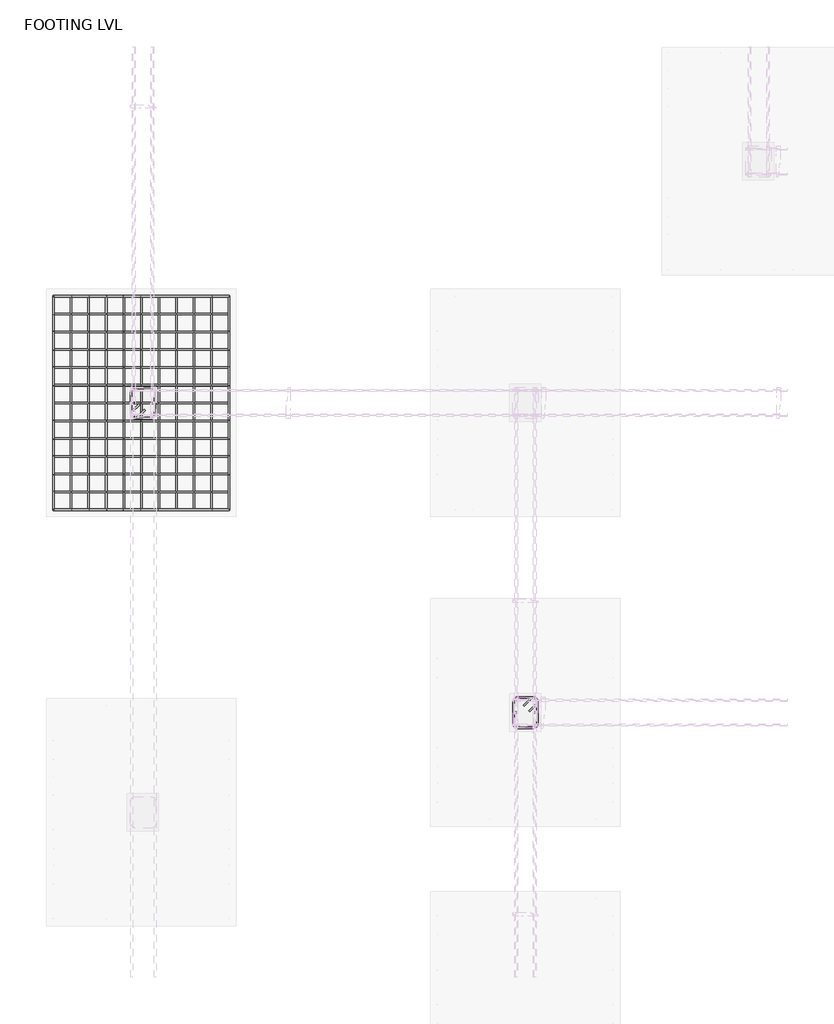
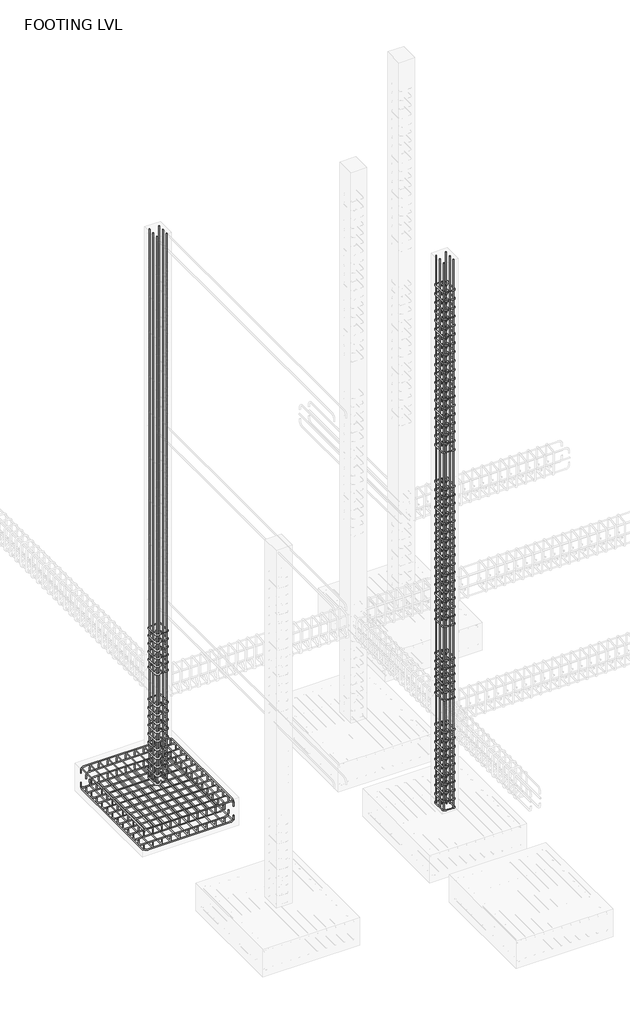
# One storey, part 4 of 16: 22 reinforcing bars.
"""IFC4 building model written with IfcOpenShell, lengths in millimetres."""

from ifc_helpers import new_model, si_unit, point, frame, origin, place, context, project, spatial, polyline, circle_curve, trimmed, segment, composite_curve, source, transform, mapped, element, save
from ifc_brep_helpers import swept_disk

model = new_model("IFC4")

# Units and contexts
model_context = context("Model", 3, world=origin())
ifc_project = project(units=[si_unit("LENGTHUNIT", "METRE", prefix="MILLI")], contexts=[model_context])

# Site, building, storey
site = spatial("IfcSite", under=ifc_project)
building = spatial("IfcBuilding", under=site)
storey = spatial("IfcBuildingStorey", under=building, Name="FOOTING LVL", Elevation=-1828.8)

# Reinforcing bars
placement = place(None, origin())
reinforcing_bar_shape = source(origin(), model_context, "Body", "SolidModel", [
    swept_disk(composite_curve([segment(polyline([(-13401.9759067, 5358.4372759, -2134.39375), (-13401.9759067, 5358.4372759, -2185.19375)]), True, "CONTINUOUS"), segment(trimmed(circle_curve(frame((-13357.5259067, 5358.4372759, -2185.19375), z_axis=(0.0, -1.0, 0.0), x_axis=(-44.44999999999891, 0.0, 0.0)), 44.45), [point((-13401.9759067, 5358.4372759, -2185.19375))], [point((-13357.5259067, 5358.4372759, -2229.64375))], True, "CARTESIAN"), True, "CONTINUOUS"), segment(polyline([(-13357.5259067, 5358.4372759, -2229.64375), (-12035.1384067, 5358.4372759, -2229.64375)]), True, "CONTINUOUS"), segment(trimmed(circle_curve(frame((-12035.1384067, 5358.4372759, -2185.19375), z_axis=(0.0, -1.0, 0.0), x_axis=(0.0, 0.0, -44.45000000000027)), 44.45), [point((-12035.1384067, 5358.4372759, -2229.64375))], [point((-11990.6884067, 5358.4372759, -2185.19375))], True, "CARTESIAN"), True, "CONTINUOUS"), segment(polyline([(-11990.6884067, 5358.4372759, -2185.19375), (-11990.6884067, 5358.4372759, -2134.39375)]), True, "CONTINUOUS")], self_intersect=False), 6.35),
])
element("IfcReinforcingBar", 1, at=placement, inside=storey, context=model_context, shape_type="MappedRepresentation", body=[
    mapped(reinforcing_bar_shape, transform((0.0, 0.0, 0.0), x_axis=(1.0, 0.0, 0.0), y_axis=(0.0, 1.0, 0.0), z_axis=(0.0, 0.0, 1.0))),
    mapped(reinforcing_bar_shape, transform((0.0, 143.0072917, 0.0), x_axis=(1.0, 0.0, 0.0), y_axis=(0.0, 1.0, 0.0), z_axis=(0.0, 0.0, 1.0))),
    mapped(reinforcing_bar_shape, transform((0.0, 286.0145833, 0.0), x_axis=(1.0, 0.0, 0.0), y_axis=(0.0, 1.0, 0.0), z_axis=(0.0, 0.0, 1.0))),
    mapped(reinforcing_bar_shape, transform((0.0, 429.021875, 0.0), x_axis=(1.0, 0.0, 0.0), y_axis=(0.0, 1.0, 0.0), z_axis=(0.0, 0.0, 1.0))),
    mapped(reinforcing_bar_shape, transform((0.0, 572.0291667, 0.0), x_axis=(1.0, 0.0, 0.0), y_axis=(0.0, 1.0, 0.0), z_axis=(0.0, 0.0, 1.0))),
    mapped(reinforcing_bar_shape, transform((0.0, 715.0364583, 0.0), x_axis=(1.0, 0.0, 0.0), y_axis=(0.0, 1.0, 0.0), z_axis=(0.0, 0.0, 1.0))),
    mapped(reinforcing_bar_shape, transform((0.0, 858.04375, 0.0), x_axis=(1.0, 0.0, 0.0), y_axis=(0.0, 1.0, 0.0), z_axis=(0.0, 0.0, 1.0))),
    mapped(reinforcing_bar_shape, transform((0.0, 1001.0510417, 0.0), x_axis=(1.0, 0.0, 0.0), y_axis=(0.0, 1.0, 0.0), z_axis=(0.0, 0.0, 1.0))),
    mapped(reinforcing_bar_shape, transform((0.0, 1144.0583333, 0.0), x_axis=(1.0, 0.0, 0.0), y_axis=(0.0, 1.0, 0.0), z_axis=(0.0, 0.0, 1.0))),
    mapped(reinforcing_bar_shape, transform((0.0, 1287.065625, 0.0), x_axis=(1.0, 0.0, 0.0), y_axis=(0.0, 1.0, 0.0), z_axis=(0.0, 0.0, 1.0))),
    mapped(reinforcing_bar_shape, transform((0.0, 1430.0729167, 0.0), x_axis=(1.0, 0.0, 0.0), y_axis=(0.0, 1.0, 0.0), z_axis=(0.0, 0.0, 1.0))),
    mapped(reinforcing_bar_shape, transform((0.0, 1573.0802083, 0.0), x_axis=(1.0, 0.0, 0.0), y_axis=(0.0, 1.0, 0.0), z_axis=(0.0, 0.0, 1.0))),
    mapped(reinforcing_bar_shape, transform((0.0, 1716.0875, 0.0), x_axis=(1.0, 0.0, 0.0), y_axis=(0.0, 1.0, 0.0), z_axis=(0.0, 0.0, 1.0))),
])
reinforcing_bar_2_shape = source(origin(), model_context, "Body", "SolidModel", [
    swept_disk(composite_curve([segment(polyline([(-11990.6884067, 5358.4372759, -1980.40625), (-11990.6884067, 5358.4372759, -1929.60625)]), True, "CONTINUOUS"), segment(trimmed(circle_curve(frame((-12035.1384067, 5358.4372759, -1929.60625), z_axis=(0.0, -1.0, 0.0), x_axis=(44.45000000000073, 0.0, 0.0)), 44.45), [point((-11990.6884067, 5358.4372759, -1929.60625))], [point((-12035.1384067, 5358.4372759, -1885.15625))], True, "CARTESIAN"), True, "CONTINUOUS"), segment(polyline([(-12035.1384067, 5358.4372759, -1885.15625), (-13357.5259067, 5358.4372759, -1885.15625)]), True, "CONTINUOUS"), segment(trimmed(circle_curve(frame((-13357.5259067, 5358.4372759, -1929.60625), z_axis=(0.0, -1.0, 0.0), x_axis=(0.0, 0.0, 44.450000000000045)), 44.45), [point((-13357.5259067, 5358.4372759, -1885.15625))], [point((-13401.9759067, 5358.4372759, -1929.60625))], True, "CARTESIAN"), True, "CONTINUOUS"), segment(polyline([(-13401.9759067, 5358.4372759, -1929.60625), (-13401.9759067, 5358.4372759, -1980.40625)]), True, "CONTINUOUS")], self_intersect=False), 6.35),
])
element("IfcReinforcingBar", 2, at=placement, inside=storey, context=model_context, shape_type="MappedRepresentation", body=[
    mapped(reinforcing_bar_2_shape, transform((0.0, 0.0, 0.0), x_axis=(1.0, 0.0, 0.0), y_axis=(0.0, 1.0, 0.0), z_axis=(0.0, 0.0, 1.0))),
    mapped(reinforcing_bar_2_shape, transform((0.0, 143.0072917, 0.0), x_axis=(1.0, 0.0, 0.0), y_axis=(0.0, 1.0, 0.0), z_axis=(0.0, 0.0, 1.0))),
    mapped(reinforcing_bar_2_shape, transform((0.0, 286.0145833, 0.0), x_axis=(1.0, 0.0, 0.0), y_axis=(0.0, 1.0, 0.0), z_axis=(0.0, 0.0, 1.0))),
    mapped(reinforcing_bar_2_shape, transform((0.0, 429.021875, 0.0), x_axis=(1.0, 0.0, 0.0), y_axis=(0.0, 1.0, 0.0), z_axis=(0.0, 0.0, 1.0))),
    mapped(reinforcing_bar_2_shape, transform((0.0, 572.0291667, 0.0), x_axis=(1.0, 0.0, 0.0), y_axis=(0.0, 1.0, 0.0), z_axis=(0.0, 0.0, 1.0))),
    mapped(reinforcing_bar_2_shape, transform((0.0, 715.0364583, 0.0), x_axis=(1.0, 0.0, 0.0), y_axis=(0.0, 1.0, 0.0), z_axis=(0.0, 0.0, 1.0))),
    mapped(reinforcing_bar_2_shape, transform((0.0, 858.04375, 0.0), x_axis=(1.0, 0.0, 0.0), y_axis=(0.0, 1.0, 0.0), z_axis=(0.0, 0.0, 1.0))),
    mapped(reinforcing_bar_2_shape, transform((0.0, 1001.0510417, 0.0), x_axis=(1.0, 0.0, 0.0), y_axis=(0.0, 1.0, 0.0), z_axis=(0.0, 0.0, 1.0))),
    mapped(reinforcing_bar_2_shape, transform((0.0, 1144.0583333, 0.0), x_axis=(1.0, 0.0, 0.0), y_axis=(0.0, 1.0, 0.0), z_axis=(0.0, 0.0, 1.0))),
    mapped(reinforcing_bar_2_shape, transform((0.0, 1287.065625, 0.0), x_axis=(1.0, 0.0, 0.0), y_axis=(0.0, 1.0, 0.0), z_axis=(0.0, 0.0, 1.0))),
    mapped(reinforcing_bar_2_shape, transform((0.0, 1430.0729167, 0.0), x_axis=(1.0, 0.0, 0.0), y_axis=(0.0, 1.0, 0.0), z_axis=(0.0, 0.0, 1.0))),
    mapped(reinforcing_bar_2_shape, transform((0.0, 1573.0802083, 0.0), x_axis=(1.0, 0.0, 0.0), y_axis=(0.0, 1.0, 0.0), z_axis=(0.0, 0.0, 1.0))),
    mapped(reinforcing_bar_2_shape, transform((0.0, 1716.0875, 0.0), x_axis=(1.0, 0.0, 0.0), y_axis=(0.0, 1.0, 0.0), z_axis=(0.0, 0.0, 1.0))),
])
reinforcing_bar_3_shape = source(origin(), model_context, "Body", "SolidModel", [
    swept_disk(composite_curve([segment(polyline([(-11990.6884067, 7074.5247759, -1980.40625), (-11990.6884067, 7074.5247759, -1929.60625)]), True, "CONTINUOUS"), segment(trimmed(circle_curve(frame((-11990.6884067, 7030.0747759, -1929.60625), z_axis=(1.0, 0.0, 0.0), x_axis=(0.0, 44.45000000000073, 0.0)), 44.45), [point((-11990.6884067, 7074.5247759, -1929.60625))], [point((-11990.6884067, 7030.0747759, -1885.15625))], True, "CARTESIAN"), True, "CONTINUOUS"), segment(polyline([(-11990.6884067, 7030.0747759, -1885.15625), (-11990.6884067, 5402.8872759, -1885.15625)]), True, "CONTINUOUS"), segment(trimmed(circle_curve(frame((-11990.6884067, 5402.8872759, -1929.60625), z_axis=(1.0, 0.0, 0.0), x_axis=(0.0, 0.0, 44.450000000000045)), 44.45), [point((-11990.6884067, 5402.8872759, -1885.15625))], [point((-11990.6884067, 5358.4372759, -1929.60625))], True, "CARTESIAN"), True, "CONTINUOUS"), segment(polyline([(-11990.6884067, 5358.4372759, -1929.60625), (-11990.6884067, 5358.4372759, -1980.40625)]), True, "CONTINUOUS")], self_intersect=False), 6.35),
])
element("IfcReinforcingBar", 3, at=placement, inside=storey, context=model_context, shape_type="MappedRepresentation", body=[
    mapped(reinforcing_bar_3_shape, transform((0.0, 0.0, 0.0), x_axis=(1.0, 0.0, 0.0), y_axis=(0.0, 1.0, 0.0), z_axis=(0.0, 0.0, 1.0))),
    mapped(reinforcing_bar_3_shape, transform((-141.12875, 0.0, 0.0), x_axis=(1.0, 0.0, 0.0), y_axis=(0.0, 1.0, 0.0), z_axis=(0.0, 0.0, 1.0))),
    mapped(reinforcing_bar_3_shape, transform((-282.2575, 0.0, 0.0), x_axis=(1.0, 0.0, 0.0), y_axis=(0.0, 1.0, 0.0), z_axis=(0.0, 0.0, 1.0))),
    mapped(reinforcing_bar_3_shape, transform((-423.38625, 0.0, 0.0), x_axis=(1.0, 0.0, 0.0), y_axis=(0.0, 1.0, 0.0), z_axis=(0.0, 0.0, 1.0))),
    mapped(reinforcing_bar_3_shape, transform((-564.515, 0.0, 0.0), x_axis=(1.0, 0.0, 0.0), y_axis=(0.0, 1.0, 0.0), z_axis=(0.0, 0.0, 1.0))),
    mapped(reinforcing_bar_3_shape, transform((-705.64375, 0.0, 0.0), x_axis=(1.0, 0.0, 0.0), y_axis=(0.0, 1.0, 0.0), z_axis=(0.0, 0.0, 1.0))),
    mapped(reinforcing_bar_3_shape, transform((-846.7725, 0.0, 0.0), x_axis=(1.0, 0.0, 0.0), y_axis=(0.0, 1.0, 0.0), z_axis=(0.0, 0.0, 1.0))),
    mapped(reinforcing_bar_3_shape, transform((-987.90125, 0.0, 0.0), x_axis=(1.0, 0.0, 0.0), y_axis=(0.0, 1.0, 0.0), z_axis=(0.0, 0.0, 1.0))),
    mapped(reinforcing_bar_3_shape, transform((-1129.03, 0.0, 0.0), x_axis=(1.0, 0.0, 0.0), y_axis=(0.0, 1.0, 0.0), z_axis=(0.0, 0.0, 1.0))),
    mapped(reinforcing_bar_3_shape, transform((-1270.15875, 0.0, 0.0), x_axis=(1.0, 0.0, 0.0), y_axis=(0.0, 1.0, 0.0), z_axis=(0.0, 0.0, 1.0))),
    mapped(reinforcing_bar_3_shape, transform((-1411.2875, 0.0, 0.0), x_axis=(1.0, 0.0, 0.0), y_axis=(0.0, 1.0, 0.0), z_axis=(0.0, 0.0, 1.0))),
])
reinforcing_bar_4_shape = source(origin(), model_context, "Body", "SolidModel", [
    swept_disk(composite_curve([segment(polyline([(-13401.9759067, 7074.5247759, -2134.39375), (-13401.9759067, 7074.5247759, -2185.19375)]), True, "CONTINUOUS"), segment(trimmed(circle_curve(frame((-13401.9759067, 7030.0747759, -2185.19375), z_axis=(-1.0, 0.0, 0.0), x_axis=(0.0, 44.45000000000073, 0.0)), 44.45), [point((-13401.9759067, 7074.5247759, -2185.19375))], [point((-13401.9759067, 7030.0747759, -2229.64375))], True, "CARTESIAN"), True, "CONTINUOUS"), segment(polyline([(-13401.9759067, 7030.0747759, -2229.64375), (-13401.9759067, 5402.8872759, -2229.64375)]), True, "CONTINUOUS"), segment(trimmed(circle_curve(frame((-13401.9759067, 5402.8872759, -2185.19375), z_axis=(-1.0, 0.0, 0.0), x_axis=(0.0, 0.0, -44.45000000000027)), 44.45), [point((-13401.9759067, 5402.8872759, -2229.64375))], [point((-13401.9759067, 5358.4372759, -2185.19375))], True, "CARTESIAN"), True, "CONTINUOUS"), segment(polyline([(-13401.9759067, 5358.4372759, -2185.19375), (-13401.9759067, 5358.4372759, -2134.39375)]), True, "CONTINUOUS")], self_intersect=False), 6.35),
])
element("IfcReinforcingBar", 4, at=placement, inside=storey, context=model_context, shape_type="MappedRepresentation", body=[
    mapped(reinforcing_bar_4_shape, transform((0.0, 0.0, 0.0), x_axis=(1.0, 0.0, 0.0), y_axis=(0.0, 1.0, 0.0), z_axis=(0.0, 0.0, 1.0))),
    mapped(reinforcing_bar_4_shape, transform((141.12875, 0.0, 0.0), x_axis=(1.0, 0.0, 0.0), y_axis=(0.0, 1.0, 0.0), z_axis=(0.0, 0.0, 1.0))),
    mapped(reinforcing_bar_4_shape, transform((282.2575, 0.0, 0.0), x_axis=(1.0, 0.0, 0.0), y_axis=(0.0, 1.0, 0.0), z_axis=(0.0, 0.0, 1.0))),
    mapped(reinforcing_bar_4_shape, transform((423.38625, 0.0, 0.0), x_axis=(1.0, 0.0, 0.0), y_axis=(0.0, 1.0, 0.0), z_axis=(0.0, 0.0, 1.0))),
    mapped(reinforcing_bar_4_shape, transform((564.515, 0.0, 0.0), x_axis=(1.0, 0.0, 0.0), y_axis=(0.0, 1.0, 0.0), z_axis=(0.0, 0.0, 1.0))),
    mapped(reinforcing_bar_4_shape, transform((705.64375, 0.0, 0.0), x_axis=(1.0, 0.0, 0.0), y_axis=(0.0, 1.0, 0.0), z_axis=(0.0, 0.0, 1.0))),
    mapped(reinforcing_bar_4_shape, transform((846.7725, 0.0, 0.0), x_axis=(1.0, 0.0, 0.0), y_axis=(0.0, 1.0, 0.0), z_axis=(0.0, 0.0, 1.0))),
    mapped(reinforcing_bar_4_shape, transform((987.90125, 0.0, 0.0), x_axis=(1.0, 0.0, 0.0), y_axis=(0.0, 1.0, 0.0), z_axis=(0.0, 0.0, 1.0))),
    mapped(reinforcing_bar_4_shape, transform((1129.03, 0.0, 0.0), x_axis=(1.0, 0.0, 0.0), y_axis=(0.0, 1.0, 0.0), z_axis=(0.0, 0.0, 1.0))),
    mapped(reinforcing_bar_4_shape, transform((1270.15875, 0.0, 0.0), x_axis=(1.0, 0.0, 0.0), y_axis=(0.0, 1.0, 0.0), z_axis=(0.0, 0.0, 1.0))),
    mapped(reinforcing_bar_4_shape, transform((1411.2875, 0.0, 0.0), x_axis=(1.0, 0.0, 0.0), y_axis=(0.0, 1.0, 0.0), z_axis=(0.0, 0.0, 1.0))),
])
reinforcing_bar_5_shape = source(origin(), model_context, "Body", "SolidModel", [
    swept_disk(composite_curve([segment(polyline([(-12714.355274, 6204.4997897, -1797.446875), (-12769.2202725, 6149.6347912, -1797.446875)]), True, "CONTINUOUS"), segment(trimmed(circle_curve(frame((-12746.7696322, 6127.1841509, -1797.446875), z_axis=(0.0, 0.0, 1.0), x_axis=(-22.450640300001396, 22.450640300000487, 0.0)), 31.75), [point((-12769.2202725, 6149.6347912, -1797.446875))], [point((-12746.7696322, 6095.4341509, -1797.446875))], True, "CARTESIAN"), True, "CONTINUOUS"), segment(polyline([(-12746.7696322, 6095.4341509, -1797.446875), (-12618.9758822, 6095.4341509, -1797.446875)]), True, "CONTINUOUS"), segment(trimmed(circle_curve(frame((-12618.9758822, 6127.1841509, -1797.446875), z_axis=(0.0, 0.0, 1.0), x_axis=(0.0, -31.75, 0.0)), 31.75), [point((-12618.9758822, 6095.4341509, -1797.446875))], [point((-12587.2258822, 6127.1841509, -1797.446875))], True, "CARTESIAN"), True, "CONTINUOUS"), segment(polyline([(-12587.2258822, 6127.1841509, -1797.446875), (-12587.2258822, 6305.7779009, -1797.446875)]), True, "CONTINUOUS"), segment(trimmed(circle_curve(frame((-12618.9061414, 6305.7779009, -1799.5501287), z_axis=(-0.06624421176864072, 0.0, 0.9978034397651431), x_axis=(31.680259200000364, 0.0, 2.1032536999998683)), 31.75), [point((-12587.2258822, 6305.7779009, -1797.446875))], [point((-12618.9061414, 6337.5279009, -1799.5501287))], True, "CARTESIAN"), True, "CONTINUOUS"), segment(polyline([(-12618.9061414, 6337.5279009, -1799.5501287), (-12746.839373, 6337.5279009, -1808.0436213)]), True, "CONTINUOUS"), segment(trimmed(circle_curve(frame((-12746.839373, 6305.7779009, -1808.0436213), z_axis=(-0.06624421176864072, 0.0, 0.9978034397651431), x_axis=(0.0, 31.75, 0.0)), 31.75), [point((-12746.839373, 6337.5279009, -1808.0436213))], [point((-12778.5196322, 6305.7779009, -1810.146875))], True, "CARTESIAN"), True, "CONTINUOUS"), segment(polyline([(-12778.5196322, 6305.7779009, -1810.146875), (-12778.5196322, 6127.1841509, -1810.146875)]), True, "CONTINUOUS"), segment(trimmed(circle_curve(frame((-12746.7696322, 6127.1841509, -1810.146875), z_axis=(0.0, 0.0, 1.0), x_axis=(-31.75, 0.0, 0.0)), 31.75), [point((-12778.5196322, 6127.1841509, -1810.146875))], [point((-12724.3189919, 6104.7335106, -1810.146875))], True, "CARTESIAN"), True, "CONTINUOUS"), segment(polyline([(-12724.3189919, 6104.7335106, -1810.146875), (-12669.4539934, 6159.5985091, -1810.146875)]), True, "CONTINUOUS")], self_intersect=False), 6.35),
])
element("IfcReinforcingBar", 5, at=placement, inside=storey, context=model_context, shape_type="MappedRepresentation", body=[
    mapped(reinforcing_bar_5_shape, transform((0.0, 0.0, 0.0), x_axis=(1.0, 0.0, 0.0), y_axis=(0.0, 1.0, 0.0), z_axis=(0.0, 0.0, 1.0))),
    mapped(reinforcing_bar_5_shape, transform((0.0, 0.0, 144.2276574), x_axis=(1.0, 0.0, 0.0), y_axis=(0.0, 1.0, 0.0), z_axis=(0.0, 0.0, 1.0))),
    mapped(reinforcing_bar_5_shape, transform((0.0, 0.0, 288.4553149), x_axis=(1.0, 0.0, 0.0), y_axis=(0.0, 1.0, 0.0), z_axis=(0.0, 0.0, 1.0))),
    mapped(reinforcing_bar_5_shape, transform((0.0, 0.0, 432.6829723), x_axis=(1.0, 0.0, 0.0), y_axis=(0.0, 1.0, 0.0), z_axis=(0.0, 0.0, 1.0))),
    mapped(reinforcing_bar_5_shape, transform((0.0, 0.0, 576.9106298), x_axis=(1.0, 0.0, 0.0), y_axis=(0.0, 1.0, 0.0), z_axis=(0.0, 0.0, 1.0))),
    mapped(reinforcing_bar_5_shape, transform((0.0, 0.0, 721.1382872), x_axis=(1.0, 0.0, 0.0), y_axis=(0.0, 1.0, 0.0), z_axis=(0.0, 0.0, 1.0))),
    mapped(reinforcing_bar_5_shape, transform((0.0, 0.0, 865.3659446), x_axis=(1.0, 0.0, 0.0), y_axis=(0.0, 1.0, 0.0), z_axis=(0.0, 0.0, 1.0))),
    mapped(reinforcing_bar_5_shape, transform((0.0, 0.0, 1009.5936021), x_axis=(1.0, 0.0, 0.0), y_axis=(0.0, 1.0, 0.0), z_axis=(0.0, 0.0, 1.0))),
    mapped(reinforcing_bar_5_shape, transform((0.0, 0.0, 1153.8212595), x_axis=(1.0, 0.0, 0.0), y_axis=(0.0, 1.0, 0.0), z_axis=(0.0, 0.0, 1.0))),
    mapped(reinforcing_bar_5_shape, transform((0.0, 0.0, 1298.048917), x_axis=(1.0, 0.0, 0.0), y_axis=(0.0, 1.0, 0.0), z_axis=(0.0, 0.0, 1.0))),
])
element("IfcReinforcingBar", 6, at=placement, inside=storey, context=model_context, shape_type="SolidModel", body=[
    swept_disk(composite_curve([segment(polyline([(-12760.2400164, 6113.7137667, -1803.796875), (-12760.2400164, 6113.7137667, 7290.196875)]), True, "CONTINUOUS")], self_intersect=False), 6.35),
])
element("IfcReinforcingBar", 7, at=placement, inside=storey, context=model_context, shape_type="SolidModel", body=[
    swept_disk(composite_curve([segment(polyline([(-12605.505498, 6113.7137667, -1803.796875), (-12605.505498, 6113.7137667, 7290.196875)]), True, "CONTINUOUS")], self_intersect=False), 6.35),
])
element("IfcReinforcingBar", 8, at=placement, inside=storey, context=model_context, shape_type="SolidModel", body=[
    swept_disk(composite_curve([segment(polyline([(-12760.2400164, 6319.2482851, -1803.796875), (-12760.2400164, 6319.2482851, 7290.196875)]), True, "CONTINUOUS")], self_intersect=False), 6.35),
])
element("IfcReinforcingBar", 9, at=placement, inside=storey, context=model_context, shape_type="SolidModel", body=[
    swept_disk(composite_curve([segment(polyline([(-12605.505498, 6319.2482851, -1803.796875), (-12605.505498, 6319.2482851, 7290.196875)]), True, "CONTINUOUS")], self_intersect=False), 6.35),
])
element("IfcReinforcingBar", 10, at=placement, inside=storey, context=model_context, shape_type="SolidModel", body=[
    swept_disk(composite_curve([segment(polyline([(-12760.2400164, 6216.4810259, -1803.796875), (-12760.2400164, 6216.4810259, 7290.196875)]), True, "CONTINUOUS")], self_intersect=False), 6.35),
])
element("IfcReinforcingBar", 11, at=placement, inside=storey, context=model_context, shape_type="SolidModel", body=[
    swept_disk(composite_curve([segment(polyline([(-12605.505498, 6216.4810259, -1803.796875), (-12605.505498, 6216.4810259, 7290.196875)]), True, "CONTINUOUS")], self_intersect=False), 6.35),
])
reinforcing_bar_6_shape = source(origin(), model_context, "Body", "SolidModel", [
    swept_disk(composite_curve([segment(polyline([(-12714.355274, 6204.4997897, 31.353125), (-12769.2202725, 6149.6347912, 31.353125)]), True, "CONTINUOUS"), segment(trimmed(circle_curve(frame((-12746.7696322, 6127.1841509, 31.353125), z_axis=(0.0, 0.0, 1.0), x_axis=(-22.450640300001396, 22.450640300000487, 0.0)), 31.75), [point((-12769.2202725, 6149.6347912, 31.353125))], [point((-12746.7696322, 6095.4341509, 31.353125))], True, "CARTESIAN"), True, "CONTINUOUS"), segment(polyline([(-12746.7696322, 6095.4341509, 31.353125), (-12618.9758822, 6095.4341509, 31.353125)]), True, "CONTINUOUS"), segment(trimmed(circle_curve(frame((-12618.9758822, 6127.1841509, 31.353125), z_axis=(0.0, 0.0, 1.0), x_axis=(0.0, -31.75, 0.0)), 31.75), [point((-12618.9758822, 6095.4341509, 31.353125))], [point((-12587.2258822, 6127.1841509, 31.353125))], True, "CARTESIAN"), True, "CONTINUOUS"), segment(polyline([(-12587.2258822, 6127.1841509, 31.353125), (-12587.2258822, 6305.7779009, 31.353125)]), True, "CONTINUOUS"), segment(trimmed(circle_curve(frame((-12618.9061414, 6305.7779009, 29.2498713), z_axis=(-0.06624421176864072, 0.0, 0.9978034397651431), x_axis=(31.680259200000364, 0.0, 2.1032537)), 31.75), [point((-12587.2258822, 6305.7779009, 31.353125))], [point((-12618.9061414, 6337.5279009, 29.2498713))], True, "CARTESIAN"), True, "CONTINUOUS"), segment(polyline([(-12618.9061414, 6337.5279009, 29.2498713), (-12746.839373, 6337.5279009, 20.7563787)]), True, "CONTINUOUS"), segment(trimmed(circle_curve(frame((-12746.839373, 6305.7779009, 20.7563787), z_axis=(-0.06624421176864072, 0.0, 0.9978034397651431), x_axis=(0.0, 31.75, 0.0)), 31.75), [point((-12746.839373, 6337.5279009, 20.7563787))], [point((-12778.5196322, 6305.7779009, 18.653125))], True, "CARTESIAN"), True, "CONTINUOUS"), segment(polyline([(-12778.5196322, 6305.7779009, 18.653125), (-12778.5196322, 6127.1841509, 18.653125)]), True, "CONTINUOUS"), segment(trimmed(circle_curve(frame((-12746.7696322, 6127.1841509, 18.653125), z_axis=(0.0, 0.0, 1.0), x_axis=(-31.75, 0.0, 0.0)), 31.75), [point((-12778.5196322, 6127.1841509, 18.653125))], [point((-12724.3189919, 6104.7335106, 18.653125))], True, "CARTESIAN"), True, "CONTINUOUS"), segment(polyline([(-12724.3189919, 6104.7335106, 18.653125), (-12669.4539934, 6159.5985091, 18.653125)]), True, "CONTINUOUS")], self_intersect=False), 6.35),
])
element("IfcReinforcingBar", 12, at=placement, inside=storey, context=model_context, shape_type="MappedRepresentation", body=[
    mapped(reinforcing_bar_6_shape, transform((0.0, 0.0, 0.0), x_axis=(1.0, 0.0, 0.0), y_axis=(0.0, 1.0, 0.0), z_axis=(0.0, 0.0, 1.0))),
    mapped(reinforcing_bar_6_shape, transform((0.0, 0.0, 130.6477176), x_axis=(1.0, 0.0, 0.0), y_axis=(0.0, 1.0, 0.0), z_axis=(0.0, 0.0, 1.0))),
    mapped(reinforcing_bar_6_shape, transform((0.0, 0.0, 261.2954352), x_axis=(1.0, 0.0, 0.0), y_axis=(0.0, 1.0, 0.0), z_axis=(0.0, 0.0, 1.0))),
    mapped(reinforcing_bar_6_shape, transform((0.0, 0.0, 391.9431528), x_axis=(1.0, 0.0, 0.0), y_axis=(0.0, 1.0, 0.0), z_axis=(0.0, 0.0, 1.0))),
    mapped(reinforcing_bar_6_shape, transform((0.0, 0.0, 522.5908704), x_axis=(1.0, 0.0, 0.0), y_axis=(0.0, 1.0, 0.0), z_axis=(0.0, 0.0, 1.0))),
    mapped(reinforcing_bar_6_shape, transform((0.0, 0.0, 653.238588), x_axis=(1.0, 0.0, 0.0), y_axis=(0.0, 1.0, 0.0), z_axis=(0.0, 0.0, 1.0))),
])
reinforcing_bar_7_shape = source(origin(), model_context, "Body", "SolidModel", [
    swept_disk(composite_curve([segment(polyline([(-9577.9902404, 3739.2622621, -1797.446875), (-9523.1252419, 3794.1272606, -1797.446875)]), True, "CONTINUOUS"), segment(trimmed(circle_curve(frame((-9545.5758822, 3816.5779009, -1797.446875), z_axis=(0.0, 0.0, 1.0), x_axis=(22.450640300001396, -22.450640299999577, 0.0)), 31.75), [point((-9523.1252419, 3794.1272606, -1797.446875))], [point((-9545.5758822, 3848.3279009, -1797.446875))], True, "CARTESIAN"), True, "CONTINUOUS"), segment(polyline([(-9545.5758822, 3848.3279009, -1797.446875), (-9673.3696322, 3848.3279009, -1797.446875)]), True, "CONTINUOUS"), segment(trimmed(circle_curve(frame((-9673.3696322, 3816.5779009, -1797.446875), z_axis=(0.0, 0.0, 1.0), x_axis=(0.0, 31.75, 0.0)), 31.75), [point((-9673.3696322, 3848.3279009, -1797.446875))], [point((-9705.1196322, 3816.5779009, -1797.446875))], True, "CARTESIAN"), True, "CONTINUOUS"), segment(polyline([(-9705.1196322, 3816.5779009, -1797.446875), (-9705.1196322, 3637.9841509, -1797.446875)]), True, "CONTINUOUS"), segment(trimmed(circle_curve(frame((-9673.439373, 3637.9841509, -1799.5501287), z_axis=(0.06624421176864072, 0.0, 0.9978034397651431), x_axis=(-31.680259200000364, 0.0, 2.1032536999998683)), 31.75), [point((-9705.1196322, 3637.9841509, -1797.446875))], [point((-9673.439373, 3606.2341509, -1799.5501287))], True, "CARTESIAN"), True, "CONTINUOUS"), segment(polyline([(-9673.439373, 3606.2341509, -1799.5501287), (-9545.5061414, 3606.2341509, -1808.0436213)]), True, "CONTINUOUS"), segment(trimmed(circle_curve(frame((-9545.5061414, 3637.9841509, -1808.0436213), z_axis=(0.06624421176864072, 0.0, 0.9978034397651431), x_axis=(0.0, -31.75, 0.0)), 31.75), [point((-9545.5061414, 3606.2341509, -1808.0436213))], [point((-9513.8258822, 3637.9841509, -1810.146875))], True, "CARTESIAN"), True, "CONTINUOUS"), segment(polyline([(-9513.8258822, 3637.9841509, -1810.146875), (-9513.8258822, 3816.5779009, -1810.146875)]), True, "CONTINUOUS"), segment(trimmed(circle_curve(frame((-9545.5758822, 3816.5779009, -1810.146875), z_axis=(0.0, 0.0, 1.0), x_axis=(31.75, 0.0, 0.0)), 31.75), [point((-9513.8258822, 3816.5779009, -1810.146875))], [point((-9568.0265225, 3839.0285412, -1810.146875))], True, "CARTESIAN"), True, "CONTINUOUS"), segment(polyline([(-9568.0265225, 3839.0285412, -1810.146875), (-9622.891521, 3784.1635427, -1810.146875)]), True, "CONTINUOUS")], self_intersect=False), 6.35),
])
element("IfcReinforcingBar", 13, at=placement, inside=storey, context=model_context, shape_type="MappedRepresentation", body=[
    mapped(reinforcing_bar_7_shape, transform((0.0, 0.0, 0.0), x_axis=(1.0, 0.0, 0.0), y_axis=(0.0, 1.0, 0.0), z_axis=(0.0, 0.0, 1.0))),
    mapped(reinforcing_bar_7_shape, transform((0.0, 0.0, 144.2276574), x_axis=(1.0, 0.0, 0.0), y_axis=(0.0, 1.0, 0.0), z_axis=(0.0, 0.0, 1.0))),
    mapped(reinforcing_bar_7_shape, transform((0.0, 0.0, 288.4553149), x_axis=(1.0, 0.0, 0.0), y_axis=(0.0, 1.0, 0.0), z_axis=(0.0, 0.0, 1.0))),
    mapped(reinforcing_bar_7_shape, transform((0.0, 0.0, 432.6829723), x_axis=(1.0, 0.0, 0.0), y_axis=(0.0, 1.0, 0.0), z_axis=(0.0, 0.0, 1.0))),
    mapped(reinforcing_bar_7_shape, transform((0.0, 0.0, 576.9106298), x_axis=(1.0, 0.0, 0.0), y_axis=(0.0, 1.0, 0.0), z_axis=(0.0, 0.0, 1.0))),
    mapped(reinforcing_bar_7_shape, transform((0.0, 0.0, 721.1382872), x_axis=(1.0, 0.0, 0.0), y_axis=(0.0, 1.0, 0.0), z_axis=(0.0, 0.0, 1.0))),
    mapped(reinforcing_bar_7_shape, transform((0.0, 0.0, 865.3659446), x_axis=(1.0, 0.0, 0.0), y_axis=(0.0, 1.0, 0.0), z_axis=(0.0, 0.0, 1.0))),
    mapped(reinforcing_bar_7_shape, transform((0.0, 0.0, 1009.5936021), x_axis=(1.0, 0.0, 0.0), y_axis=(0.0, 1.0, 0.0), z_axis=(0.0, 0.0, 1.0))),
    mapped(reinforcing_bar_7_shape, transform((0.0, 0.0, 1153.8212595), x_axis=(1.0, 0.0, 0.0), y_axis=(0.0, 1.0, 0.0), z_axis=(0.0, 0.0, 1.0))),
    mapped(reinforcing_bar_7_shape, transform((0.0, 0.0, 1298.048917), x_axis=(1.0, 0.0, 0.0), y_axis=(0.0, 1.0, 0.0), z_axis=(0.0, 0.0, 1.0))),
])
element("IfcReinforcingBar", 14, at=placement, inside=storey, context=model_context, shape_type="SolidModel", body=[
    swept_disk(composite_curve([segment(polyline([(-9532.105498, 3830.0482851, -1803.796875), (-9532.105498, 3830.0482851, 7290.196875)]), True, "CONTINUOUS")], self_intersect=False), 6.35),
])
element("IfcReinforcingBar", 15, at=placement, inside=storey, context=model_context, shape_type="SolidModel", body=[
    swept_disk(composite_curve([segment(polyline([(-9686.8400164, 3830.0482851, -1803.796875), (-9686.8400164, 3830.0482851, 7290.196875)]), True, "CONTINUOUS")], self_intersect=False), 6.35),
])
element("IfcReinforcingBar", 16, at=placement, inside=storey, context=model_context, shape_type="SolidModel", body=[
    swept_disk(composite_curve([segment(polyline([(-9532.105498, 3624.5137667, -1803.796875), (-9532.105498, 3624.5137667, 7290.196875)]), True, "CONTINUOUS")], self_intersect=False), 6.35),
])
element("IfcReinforcingBar", 17, at=placement, inside=storey, context=model_context, shape_type="SolidModel", body=[
    swept_disk(composite_curve([segment(polyline([(-9686.8400164, 3624.5137667, -1803.796875), (-9686.8400164, 3624.5137667, 7290.196875)]), True, "CONTINUOUS")], self_intersect=False), 6.35),
])
element("IfcReinforcingBar", 18, at=placement, inside=storey, context=model_context, shape_type="SolidModel", body=[
    swept_disk(composite_curve([segment(polyline([(-9532.105498, 3727.2810259, -1803.796875), (-9532.105498, 3727.2810259, 7290.196875)]), True, "CONTINUOUS")], self_intersect=False), 6.35),
])
element("IfcReinforcingBar", 19, at=placement, inside=storey, context=model_context, shape_type="SolidModel", body=[
    swept_disk(composite_curve([segment(polyline([(-9686.8400164, 3727.2810259, -1803.796875), (-9686.8400164, 3727.2810259, 7290.196875)]), True, "CONTINUOUS")], self_intersect=False), 6.35),
])
reinforcing_bar_8_shape = source(origin(), model_context, "Body", "SolidModel", [
    swept_disk(composite_curve([segment(polyline([(-9577.9902404, 3739.2622621, 31.353125), (-9523.1252419, 3794.1272606, 31.353125)]), True, "CONTINUOUS"), segment(trimmed(circle_curve(frame((-9545.5758822, 3816.5779009, 31.353125), z_axis=(0.0, 0.0, 1.0), x_axis=(22.450640300001396, -22.450640299999577, 0.0)), 31.75), [point((-9523.1252419, 3794.1272606, 31.353125))], [point((-9545.5758822, 3848.3279009, 31.353125))], True, "CARTESIAN"), True, "CONTINUOUS"), segment(polyline([(-9545.5758822, 3848.3279009, 31.353125), (-9673.3696322, 3848.3279009, 31.353125)]), True, "CONTINUOUS"), segment(trimmed(circle_curve(frame((-9673.3696322, 3816.5779009, 31.353125), z_axis=(0.0, 0.0, 1.0), x_axis=(0.0, 31.75, 0.0)), 31.75), [point((-9673.3696322, 3848.3279009, 31.353125))], [point((-9705.1196322, 3816.5779009, 31.353125))], True, "CARTESIAN"), True, "CONTINUOUS"), segment(polyline([(-9705.1196322, 3816.5779009, 31.353125), (-9705.1196322, 3637.9841509, 31.353125)]), True, "CONTINUOUS"), segment(trimmed(circle_curve(frame((-9673.439373, 3637.9841509, 29.2498713), z_axis=(0.06624421176864072, 0.0, 0.9978034397651431), x_axis=(-31.680259200000364, 0.0, 2.1032537)), 31.75), [point((-9705.1196322, 3637.9841509, 31.353125))], [point((-9673.439373, 3606.2341509, 29.2498713))], True, "CARTESIAN"), True, "CONTINUOUS"), segment(polyline([(-9673.439373, 3606.2341509, 29.2498713), (-9545.5061414, 3606.2341509, 20.7563787)]), True, "CONTINUOUS"), segment(trimmed(circle_curve(frame((-9545.5061414, 3637.9841509, 20.7563787), z_axis=(0.06624421176864072, 0.0, 0.9978034397651431), x_axis=(0.0, -31.75, 0.0)), 31.75), [point((-9545.5061414, 3606.2341509, 20.7563787))], [point((-9513.8258822, 3637.9841509, 18.653125))], True, "CARTESIAN"), True, "CONTINUOUS"), segment(polyline([(-9513.8258822, 3637.9841509, 18.653125), (-9513.8258822, 3816.5779009, 18.653125)]), True, "CONTINUOUS"), segment(trimmed(circle_curve(frame((-9545.5758822, 3816.5779009, 18.653125), z_axis=(0.0, 0.0, 1.0), x_axis=(31.75, 0.0, 0.0)), 31.75), [point((-9513.8258822, 3816.5779009, 18.653125))], [point((-9568.0265225, 3839.0285412, 18.653125))], True, "CARTESIAN"), True, "CONTINUOUS"), segment(polyline([(-9568.0265225, 3839.0285412, 18.653125), (-9622.891521, 3784.1635427, 18.653125)]), True, "CONTINUOUS")], self_intersect=False), 6.35),
])
element("IfcReinforcingBar", 20, at=placement, inside=storey, context=model_context, shape_type="MappedRepresentation", body=[
    mapped(reinforcing_bar_8_shape, transform((0.0, 0.0, 0.0), x_axis=(1.0, 0.0, 0.0), y_axis=(0.0, 1.0, 0.0), z_axis=(0.0, 0.0, 1.0))),
    mapped(reinforcing_bar_8_shape, transform((0.0, 0.0, 130.6477176), x_axis=(1.0, 0.0, 0.0), y_axis=(0.0, 1.0, 0.0), z_axis=(0.0, 0.0, 1.0))),
    mapped(reinforcing_bar_8_shape, transform((0.0, 0.0, 261.2954352), x_axis=(1.0, 0.0, 0.0), y_axis=(0.0, 1.0, 0.0), z_axis=(0.0, 0.0, 1.0))),
    mapped(reinforcing_bar_8_shape, transform((0.0, 0.0, 391.9431528), x_axis=(1.0, 0.0, 0.0), y_axis=(0.0, 1.0, 0.0), z_axis=(0.0, 0.0, 1.0))),
    mapped(reinforcing_bar_8_shape, transform((0.0, 0.0, 522.5908704), x_axis=(1.0, 0.0, 0.0), y_axis=(0.0, 1.0, 0.0), z_axis=(0.0, 0.0, 1.0))),
    mapped(reinforcing_bar_8_shape, transform((0.0, 0.0, 653.238588), x_axis=(1.0, 0.0, 0.0), y_axis=(0.0, 1.0, 0.0), z_axis=(0.0, 0.0, 1.0))),
])
reinforcing_bar_9_shape = source(origin(), model_context, "Body", "SolidModel", [
    swept_disk(composite_curve([segment(polyline([(-9577.9902404, 3739.2622621, 1250.553125), (-9523.1252419, 3794.1272606, 1250.553125)]), True, "CONTINUOUS"), segment(trimmed(circle_curve(frame((-9545.5758822, 3816.5779009, 1250.553125), z_axis=(0.0, 0.0, 1.0), x_axis=(22.450640300001396, -22.450640299999577, 0.0)), 31.75), [point((-9523.1252419, 3794.1272606, 1250.553125))], [point((-9545.5758822, 3848.3279009, 1250.553125))], True, "CARTESIAN"), True, "CONTINUOUS"), segment(polyline([(-9545.5758822, 3848.3279009, 1250.553125), (-9673.3696322, 3848.3279009, 1250.553125)]), True, "CONTINUOUS"), segment(trimmed(circle_curve(frame((-9673.3696322, 3816.5779009, 1250.553125), z_axis=(0.0, 0.0, 1.0), x_axis=(0.0, 31.75, 0.0)), 31.75), [point((-9673.3696322, 3848.3279009, 1250.553125))], [point((-9705.1196322, 3816.5779009, 1250.553125))], True, "CARTESIAN"), True, "CONTINUOUS"), segment(polyline([(-9705.1196322, 3816.5779009, 1250.553125), (-9705.1196322, 3637.9841509, 1250.553125)]), True, "CONTINUOUS"), segment(trimmed(circle_curve(frame((-9673.439373, 3637.9841509, 1248.4498713), z_axis=(0.06624421176864072, 0.0, 0.9978034397651431), x_axis=(-31.680259200000364, 0.0, 2.1032536999998683)), 31.75), [point((-9705.1196322, 3637.9841509, 1250.553125))], [point((-9673.439373, 3606.2341509, 1248.4498713))], True, "CARTESIAN"), True, "CONTINUOUS"), segment(polyline([(-9673.439373, 3606.2341509, 1248.4498713), (-9545.5061414, 3606.2341509, 1239.9563787)]), True, "CONTINUOUS"), segment(trimmed(circle_curve(frame((-9545.5061414, 3637.9841509, 1239.9563787), z_axis=(0.06624421176864072, 0.0, 0.9978034397651431), x_axis=(0.0, -31.75, 0.0)), 31.75), [point((-9545.5061414, 3606.2341509, 1239.9563787))], [point((-9513.8258822, 3637.9841509, 1237.853125))], True, "CARTESIAN"), True, "CONTINUOUS"), segment(polyline([(-9513.8258822, 3637.9841509, 1237.853125), (-9513.8258822, 3816.5779009, 1237.853125)]), True, "CONTINUOUS"), segment(trimmed(circle_curve(frame((-9545.5758822, 3816.5779009, 1237.853125), z_axis=(0.0, 0.0, 1.0), x_axis=(31.75, 0.0, 0.0)), 31.75), [point((-9513.8258822, 3816.5779009, 1237.853125))], [point((-9568.0265225, 3839.0285412, 1237.853125))], True, "CARTESIAN"), True, "CONTINUOUS"), segment(polyline([(-9568.0265225, 3839.0285412, 1237.853125), (-9622.891521, 3784.1635427, 1237.853125)]), True, "CONTINUOUS")], self_intersect=False), 6.35),
])
element("IfcReinforcingBar", 21, at=placement, inside=storey, context=model_context, shape_type="MappedRepresentation", body=[
    mapped(reinforcing_bar_9_shape, transform((0.0, 0.0, 0.0), x_axis=(1.0, 0.0, 0.0), y_axis=(0.0, 1.0, 0.0), z_axis=(0.0, 0.0, 1.0))),
    mapped(reinforcing_bar_9_shape, transform((0.0, 0.0, 142.9836687), x_axis=(1.0, 0.0, 0.0), y_axis=(0.0, 1.0, 0.0), z_axis=(0.0, 0.0, 1.0))),
    mapped(reinforcing_bar_9_shape, transform((0.0, 0.0, 285.9673374), x_axis=(1.0, 0.0, 0.0), y_axis=(0.0, 1.0, 0.0), z_axis=(0.0, 0.0, 1.0))),
    mapped(reinforcing_bar_9_shape, transform((0.0, 0.0, 428.9510061), x_axis=(1.0, 0.0, 0.0), y_axis=(0.0, 1.0, 0.0), z_axis=(0.0, 0.0, 1.0))),
    mapped(reinforcing_bar_9_shape, transform((0.0, 0.0, 571.9346748), x_axis=(1.0, 0.0, 0.0), y_axis=(0.0, 1.0, 0.0), z_axis=(0.0, 0.0, 1.0))),
    mapped(reinforcing_bar_9_shape, transform((0.0, 0.0, 714.9183435), x_axis=(1.0, 0.0, 0.0), y_axis=(0.0, 1.0, 0.0), z_axis=(0.0, 0.0, 1.0))),
    mapped(reinforcing_bar_9_shape, transform((0.0, 0.0, 857.9020122), x_axis=(1.0, 0.0, 0.0), y_axis=(0.0, 1.0, 0.0), z_axis=(0.0, 0.0, 1.0))),
    mapped(reinforcing_bar_9_shape, transform((0.0, 0.0, 1000.8856809), x_axis=(1.0, 0.0, 0.0), y_axis=(0.0, 1.0, 0.0), z_axis=(0.0, 0.0, 1.0))),
    mapped(reinforcing_bar_9_shape, transform((0.0, 0.0, 1143.8693496), x_axis=(1.0, 0.0, 0.0), y_axis=(0.0, 1.0, 0.0), z_axis=(0.0, 0.0, 1.0))),
    mapped(reinforcing_bar_9_shape, transform((0.0, 0.0, 1286.8530183), x_axis=(1.0, 0.0, 0.0), y_axis=(0.0, 1.0, 0.0), z_axis=(0.0, 0.0, 1.0))),
    mapped(reinforcing_bar_9_shape, transform((0.0, 0.0, 1429.836687), x_axis=(1.0, 0.0, 0.0), y_axis=(0.0, 1.0, 0.0), z_axis=(0.0, 0.0, 1.0))),
    mapped(reinforcing_bar_9_shape, transform((0.0, 0.0, 1572.8203557), x_axis=(1.0, 0.0, 0.0), y_axis=(0.0, 1.0, 0.0), z_axis=(0.0, 0.0, 1.0))),
    mapped(reinforcing_bar_9_shape, transform((0.0, 0.0, 1715.8040244), x_axis=(1.0, 0.0, 0.0), y_axis=(0.0, 1.0, 0.0), z_axis=(0.0, 0.0, 1.0))),
    mapped(reinforcing_bar_9_shape, transform((0.0, 0.0, 1858.7876931), x_axis=(1.0, 0.0, 0.0), y_axis=(0.0, 1.0, 0.0), z_axis=(0.0, 0.0, 1.0))),
    mapped(reinforcing_bar_9_shape, transform((0.0, 0.0, 2001.7713618), x_axis=(1.0, 0.0, 0.0), y_axis=(0.0, 1.0, 0.0), z_axis=(0.0, 0.0, 1.0))),
    mapped(reinforcing_bar_9_shape, transform((0.0, 0.0, 2144.7550305), x_axis=(1.0, 0.0, 0.0), y_axis=(0.0, 1.0, 0.0), z_axis=(0.0, 0.0, 1.0))),
    mapped(reinforcing_bar_9_shape, transform((0.0, 0.0, 2287.7386992), x_axis=(1.0, 0.0, 0.0), y_axis=(0.0, 1.0, 0.0), z_axis=(0.0, 0.0, 1.0))),
])
reinforcing_bar_10_shape = source(origin(), model_context, "Body", "SolidModel", [
    swept_disk(composite_curve([segment(polyline([(-9577.9902404, 3739.2622621, 4146.153125), (-9523.1252419, 3794.1272606, 4146.153125)]), True, "CONTINUOUS"), segment(trimmed(circle_curve(frame((-9545.5758822, 3816.5779009, 4146.153125), z_axis=(0.0, 0.0, 1.0), x_axis=(22.450640300001396, -22.450640299999577, 0.0)), 31.75), [point((-9523.1252419, 3794.1272606, 4146.153125))], [point((-9545.5758822, 3848.3279009, 4146.153125))], True, "CARTESIAN"), True, "CONTINUOUS"), segment(polyline([(-9545.5758822, 3848.3279009, 4146.153125), (-9673.3696322, 3848.3279009, 4146.153125)]), True, "CONTINUOUS"), segment(trimmed(circle_curve(frame((-9673.3696322, 3816.5779009, 4146.153125), z_axis=(0.0, 0.0, 1.0), x_axis=(0.0, 31.75, 0.0)), 31.75), [point((-9673.3696322, 3848.3279009, 4146.153125))], [point((-9705.1196322, 3816.5779009, 4146.153125))], True, "CARTESIAN"), True, "CONTINUOUS"), segment(polyline([(-9705.1196322, 3816.5779009, 4146.153125), (-9705.1196322, 3637.9841509, 4146.153125)]), True, "CONTINUOUS"), segment(trimmed(circle_curve(frame((-9673.439373, 3637.9841509, 4144.0498713), z_axis=(0.06624421176864072, 0.0, 0.9978034397651431), x_axis=(-31.680259200000364, 0.0, 2.1032537000000957)), 31.75), [point((-9705.1196322, 3637.9841509, 4146.153125))], [point((-9673.439373, 3606.2341509, 4144.0498713))], True, "CARTESIAN"), True, "CONTINUOUS"), segment(polyline([(-9673.439373, 3606.2341509, 4144.0498713), (-9545.5061414, 3606.2341509, 4135.5563787)]), True, "CONTINUOUS"), segment(trimmed(circle_curve(frame((-9545.5061414, 3637.9841509, 4135.5563787), z_axis=(0.06624421176864072, 0.0, 0.9978034397651431), x_axis=(0.0, -31.75, 0.0)), 31.75), [point((-9545.5061414, 3606.2341509, 4135.5563787))], [point((-9513.8258822, 3637.9841509, 4133.453125))], True, "CARTESIAN"), True, "CONTINUOUS"), segment(polyline([(-9513.8258822, 3637.9841509, 4133.453125), (-9513.8258822, 3816.5779009, 4133.453125)]), True, "CONTINUOUS"), segment(trimmed(circle_curve(frame((-9545.5758822, 3816.5779009, 4133.453125), z_axis=(0.0, 0.0, 1.0), x_axis=(31.75, 0.0, 0.0)), 31.75), [point((-9513.8258822, 3816.5779009, 4133.453125))], [point((-9568.0265225, 3839.0285412, 4133.453125))], True, "CARTESIAN"), True, "CONTINUOUS"), segment(polyline([(-9568.0265225, 3839.0285412, 4133.453125), (-9622.891521, 3784.1635427, 4133.453125)]), True, "CONTINUOUS")], self_intersect=False), 6.35),
])
element("IfcReinforcingBar", 22, at=placement, inside=storey, context=model_context, shape_type="MappedRepresentation", body=[
    mapped(reinforcing_bar_10_shape, transform((0.0, 0.0, 0.0), x_axis=(1.0, 0.0, 0.0), y_axis=(0.0, 1.0, 0.0), z_axis=(0.0, 0.0, 1.0))),
    mapped(reinforcing_bar_10_shape, transform((0.0, 0.0, 147.7188031), x_axis=(1.0, 0.0, 0.0), y_axis=(0.0, 1.0, 0.0), z_axis=(0.0, 0.0, 1.0))),
    mapped(reinforcing_bar_10_shape, transform((0.0, 0.0, 295.4376062), x_axis=(1.0, 0.0, 0.0), y_axis=(0.0, 1.0, 0.0), z_axis=(0.0, 0.0, 1.0))),
    mapped(reinforcing_bar_10_shape, transform((0.0, 0.0, 443.1564093), x_axis=(1.0, 0.0, 0.0), y_axis=(0.0, 1.0, 0.0), z_axis=(0.0, 0.0, 1.0))),
    mapped(reinforcing_bar_10_shape, transform((0.0, 0.0, 590.8752124), x_axis=(1.0, 0.0, 0.0), y_axis=(0.0, 1.0, 0.0), z_axis=(0.0, 0.0, 1.0))),
    mapped(reinforcing_bar_10_shape, transform((0.0, 0.0, 738.5940155), x_axis=(1.0, 0.0, 0.0), y_axis=(0.0, 1.0, 0.0), z_axis=(0.0, 0.0, 1.0))),
    mapped(reinforcing_bar_10_shape, transform((0.0, 0.0, 886.3128187), x_axis=(1.0, 0.0, 0.0), y_axis=(0.0, 1.0, 0.0), z_axis=(0.0, 0.0, 1.0))),
    mapped(reinforcing_bar_10_shape, transform((0.0, 0.0, 1034.0316218), x_axis=(1.0, 0.0, 0.0), y_axis=(0.0, 1.0, 0.0), z_axis=(0.0, 0.0, 1.0))),
    mapped(reinforcing_bar_10_shape, transform((0.0, 0.0, 1181.7504249), x_axis=(1.0, 0.0, 0.0), y_axis=(0.0, 1.0, 0.0), z_axis=(0.0, 0.0, 1.0))),
    mapped(reinforcing_bar_10_shape, transform((0.0, 0.0, 1329.469228), x_axis=(1.0, 0.0, 0.0), y_axis=(0.0, 1.0, 0.0), z_axis=(0.0, 0.0, 1.0))),
    mapped(reinforcing_bar_10_shape, transform((0.0, 0.0, 1477.1880311), x_axis=(1.0, 0.0, 0.0), y_axis=(0.0, 1.0, 0.0), z_axis=(0.0, 0.0, 1.0))),
    mapped(reinforcing_bar_10_shape, transform((0.0, 0.0, 1624.9068342), x_axis=(1.0, 0.0, 0.0), y_axis=(0.0, 1.0, 0.0), z_axis=(0.0, 0.0, 1.0))),
    mapped(reinforcing_bar_10_shape, transform((0.0, 0.0, 1772.6256373), x_axis=(1.0, 0.0, 0.0), y_axis=(0.0, 1.0, 0.0), z_axis=(0.0, 0.0, 1.0))),
    mapped(reinforcing_bar_10_shape, transform((0.0, 0.0, 1920.3444404), x_axis=(1.0, 0.0, 0.0), y_axis=(0.0, 1.0, 0.0), z_axis=(0.0, 0.0, 1.0))),
    mapped(reinforcing_bar_10_shape, transform((0.0, 0.0, 2068.0632435), x_axis=(1.0, 0.0, 0.0), y_axis=(0.0, 1.0, 0.0), z_axis=(0.0, 0.0, 1.0))),
    mapped(reinforcing_bar_10_shape, transform((0.0, 0.0, 2215.7820466), x_axis=(1.0, 0.0, 0.0), y_axis=(0.0, 1.0, 0.0), z_axis=(0.0, 0.0, 1.0))),
    mapped(reinforcing_bar_10_shape, transform((0.0, 0.0, 2363.5008497), x_axis=(1.0, 0.0, 0.0), y_axis=(0.0, 1.0, 0.0), z_axis=(0.0, 0.0, 1.0))),
    mapped(reinforcing_bar_10_shape, transform((0.0, 0.0, 2511.2196529), x_axis=(1.0, 0.0, 0.0), y_axis=(0.0, 1.0, 0.0), z_axis=(0.0, 0.0, 1.0))),
    mapped(reinforcing_bar_10_shape, transform((0.0, 0.0, 2658.938456), x_axis=(1.0, 0.0, 0.0), y_axis=(0.0, 1.0, 0.0), z_axis=(0.0, 0.0, 1.0))),
])

save(model, "model.ifc")

# Revit data of these elements
# Elements 1, 2, 3, 4, 5, 6, 7, 8, 9, 10, 11, 12, 13, 14, 15, 16, 17, 18, 19, 20, 21, 22 (IfcReinforcingBar)
#   Phase Created = New Construction
